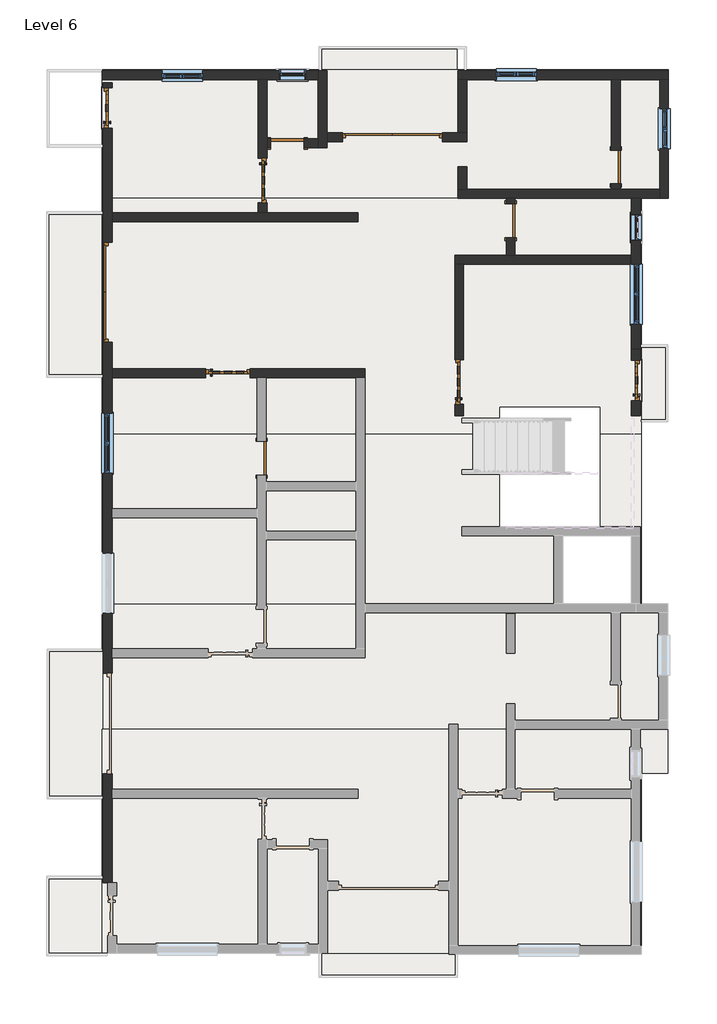
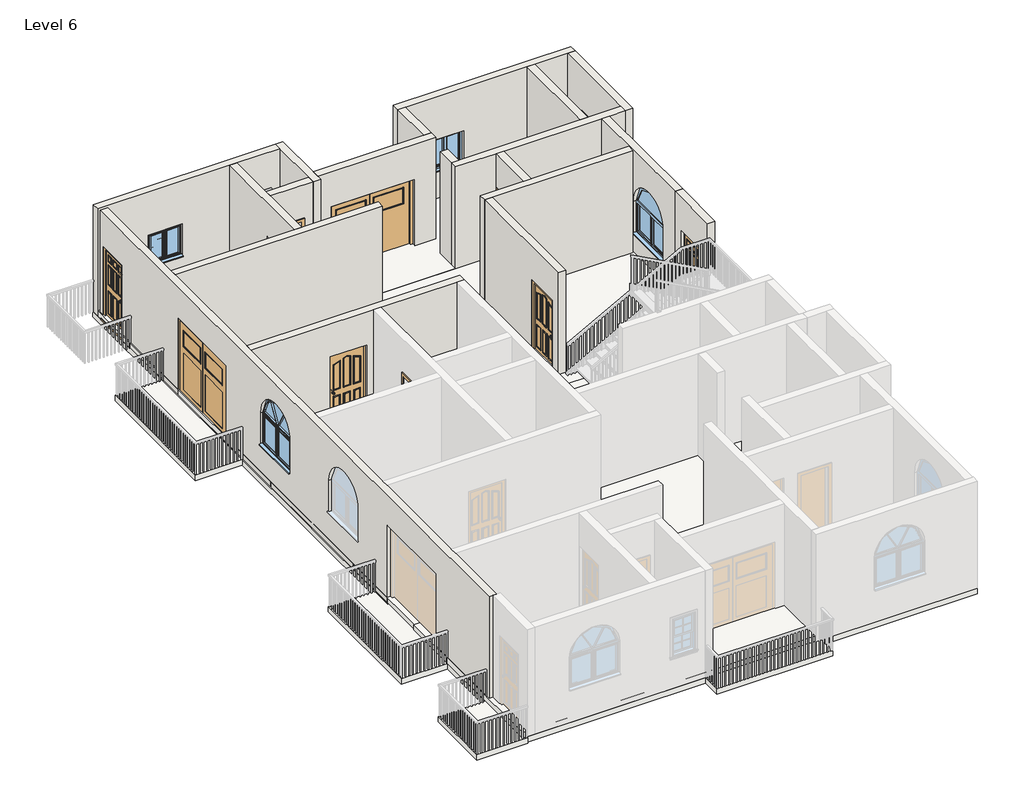
# One storey, part 2 of 7: 19 walls, 11 doors, 9 slabs, 7 windows, 5 roofs.
# Revit data of these elements (continued)
# Type "Windows_Dbl_w-Glazing_Bars : 910x910mm" (continued)
#   Frame Depth = 0' - 2.55906"
#   Default Head Height = 6' - 10.67717"
#   Cill Depth = 0' - 3.44488"
#   Cavity Closer Width = 0' - 1.9685"
#   Cavity Closer Offset from Ext = 0' - 4.03543"
#   Cavity Closer Depth = 0' - 3.34646"
#   Vis - Glazing Bars = yes
#   Vis - Cavity Closers = yes
#   Define Thermal Properties by = 1
#   Material Trim = Window Frame
#   Material Glazing Bars = Window Frame
#   Material Glass = Glass
#   Material Frame = Window Frame
#   Wall Closure = (empty or 0)
# Elements 1, 2 (IfcDoor, "Doors_ExtSgl_5 : 910x2110mm")
#   Phase Created = New Construction
#   Materials on its faces: "Door - Panel", "Door - Handle", "Door - Frame/Mullion", "Door - Glazing"
# Elements 3, 4, 5 (IfcDoor, "Doors_ExtSgl_6 : 1010x2110mm")
#   Phase Created = New Construction
#   Materials on its faces: "Door - Panel", "Door - Handle", "Door - Frame/Mullion", "Door - Glazing"
# Element 6 (IfcDoor, "Doors_Garage_Timber_Side_Hung_Glazing : 2270x2050mm")
#   Phase Created = New Construction
#   Materials on its faces: "Door - Panel", "Door - Frame/Mullion", "Door - Glazing"
# Element 7 (IfcDoor, "Doors_Garage_Timber_Side_Hung_Glazing : 2270x2200mm")
#   Phase Created = New Construction
#   Materials on its faces: "Door - Panel", "Door - Frame/Mullion", "Door - Glazing"
# Elements 8, 9, 10, 11 (IfcDoor, "Single-Flush : 30\" x 80\"")
#   Phase Created = New Construction
#   Materials on its faces: "Door - Frame", "Door - Panel"
# Elements 12, 16 (IfcRoof, "Generic - 12\"")
#   built-in parameter 1001705 = 50.5 (stored number, unit not read)
#   built-in parameter 1001710 = 33615
#   Phase Created = New Construction
#   Materials on its faces: "Default Roof", "Earth"
# Element 13 (IfcRoof, "Generic - 12\"")
#   built-in parameter 1001705 = 50.5 (stored number, unit not read)
#   built-in parameter 1001710 = 33615
#   Phase Created = New Construction
#   Materials on its faces: "Default Roof"
# Element 14 (IfcRoof, "Generic - 12\"")
#   built-in parameter 1001705 = 50.5 (stored number, unit not read)
#   built-in parameter 1001710 = 33615
#   Phase Created = New Construction
#   Materials on its faces: "Default Roof", "Concrete, Lightweight"
# Element 15 (IfcRoof, "Generic - 12\"")
#   built-in parameter 1001705 = 50.5 (stored number, unit not read)
#   built-in parameter 1001710 = 33615
#   Phase Created = New Construction
#   Materials on its faces: "Default Roof", "Wood - Stained"
# Element 17 (IfcSlab, "Generic - 12\"")
#   Height Offset From Level = 0' - 0"
#   Phase Created = New Construction
#   Materials on its faces: "Default Floor", "Concrete, Lightweight"
# Element 18 (IfcSlab, "Generic - 12\"")
#   Height Offset From Level = 0' - 0"
#   Phase Created = New Construction
#   Materials on its faces: "Default Floor", "Wood - Stained", "Earth"
# Elements 19, 21, 22, 23, 24 (IfcSlab, "Generic - 12\"")
#   Height Offset From Level = 0' - 0"
#   Phase Created = New Construction
#   Materials on its faces: "Default Floor"
# Element 20 (IfcSlab, "Generic - 12\"")
#   Height Offset From Level = 0' - 0"
#   Phase Created = New Construction
#   Materials on its faces: "Default Floor", "mm", "Brick, Soldier Course"
# Element 25 (IfcSlab, "Generic - 12\"")
#   Height Offset From Level = 0' - 0"
#   Phase Created = New Construction
#   Materials on its faces: "Default Floor", "Earth", "Concrete, Lightweight"
# Elements 26, 30 (IfcWall, "Generic - 9\" w")
#   Top Offset = 0' - 0"
#   Base Offset = 0' - 0"
#   wall height = 10' - 0"
#   Phase Created = New Construction
#   Base Constraint = Level 6
#   Top Constraint = Level 7
#   Materials on its faces: "Default Wall", "Earth"
# Element 27 (IfcWall, "Generic - 9\" w")
#   Top Offset = 0' - 0"
#   Base Offset = 0' - 0"
#   wall height = 10' - 0"
#   Phase Created = New Construction
#   Base Constraint = Level 6
#   Top Constraint = Level 7
#   Materials on its faces: "Default Wall", "Wood - Stained"
# Element 28 (IfcWall, "Generic - 9\" w")
#   Top Offset = 0' - 0"
#   Base Offset = 0' - 0"
#   wall height = 10' - 0"
#   Phase Created = New Construction
#   Base Constraint = Level 6
#   Top Constraint = Level 7
#   Materials on its faces: "Default Wall", "Grass"
# Element 29 (IfcWall, "Generic - 9\" w")
#   Top Offset = 0' - 0"
#   Base Offset = 0' - 0"
#   wall height = 10' - 0"
#   Phase Created = New Construction
#   Base Constraint = Level 6
#   Top Constraint = Level 7
#   Materials on its faces: "Default Wall", "mm"
# Elements 31, 32, 34, 36, 37, 39, 40, 41, 42, 43, 44 (IfcWall, "Generic -4.5\" p")
#   Top Offset = 0' - 0"
#   Base Offset = 0' - 0"
#   wall height = 10' - 0"
#   Phase Created = New Construction
#   Base Constraint = Level 6
#   Top Constraint = Level 7
#   Materials on its faces: "Default Wall"
# Elements 33, 38 (IfcWall, "Generic -4.5\" p")
#   Top Offset = 0' - 0"
#   Base Offset = 0' - 0"
#   wall height = 10' - 0"
#   Phase Created = New Construction
#   Base Constraint = Level 6
#   Top Constraint = Level 7
#   Materials on its faces: "Default Wall", "Earth"
# Element 35 (IfcWall, "Generic -4.5\" p")
#   Top Offset = 0' - 0"
#   Base Offset = 0' - 0"
#   wall height = 10' - 0"
#   Phase Created = New Construction
#   Base Constraint = Level 6
#   Top Constraint = Level 7
#   Materials on its faces: "Default Wall", "Oak Flooring"
# Element 45 (IfcWindow, "Window-Double-Hung : 24\" x 42\"")
#   Mark = "72"
#   Window Inset = 0' - 0"
#   Interior Wall Closure = 0' - 1 1/2"
#   Frame Extension = 0' - 1 1/4"
#   Exterior Wall Closure = 0' - 0 1/2"
#   Interior Trim Visibility = yes
#   Indicator Visibility = yes
#   Exterior Trim Visibility = yes
#   Phase Created = New Construction
#   Materials on its faces: "Wood - Stained", "Glass", "Clad - White"
# Element 46 (IfcWindow, "Window-Double-Hung : 24\" x 42\"")
#   Mark = "78"
#   Window Inset = 0' - 0"
#   Interior Wall Closure = 0' - 1 1/2"
#   Frame Extension = 0' - 1 1/4"
#   Exterior Wall Closure = 0' - 0 1/2"
#   Interior Trim Visibility = yes
#   Indicator Visibility = yes
#   Exterior Trim Visibility = yes
#   Phase Created = New Construction
#   Materials on its faces: "Wood - Stained", "Glass", "Clad - White"
# Element 47 (IfcWindow, "Windows_Arched : 1360x910mm")
#   Mark = "68"
#   Phase Created = New Construction
#   Materials on its faces: "Window Frame", "Glass"
# Element 48 (IfcWindow, "Windows_Arched : 1360x910mm")
#   Mark = "79"
#   Phase Created = New Construction
#   Materials on its faces: "Window Frame", "Glass"
# Element 49 (IfcWindow, "Windows_Dbl_w-Glazing_Bars : 910x910mm")
#   Mark = "75"
#   Phase Created = New Construction
#   Materials on its faces: "Window Frame", "Glass"
# Element 50 (IfcWindow, "Windows_Dbl_w-Glazing_Bars : 910x910mm")
#   Mark = "76"
#   Phase Created = New Construction
#   Materials on its faces: "Window Frame", "Glass"
# Element 51 (IfcWindow, "Windows_Dbl_w-Glazing_Bars : 910x910mm")
#   Mark = "77"
#   Phase Created = New Construction
#   Materials on its faces: "Window Frame", "Glass"
# Materials
#   "Door - Glazing": colour RGB 0 0 255, transparency 0.75
#   "Door - Panel": class "Wood", colour RGB 210 159 95, transparency 0, Cost = 0
#   "Door - Frame/Mullion": class "Wood", colour RGB 212 179 113, transparency 0
#   "Door - Handle": colour RGB 0 0 0, transparency 0
#   "Door - Frame": colour RGB 118 70 51, transparency 0, Cost = 0
#   "Wood - Stained": class "Wood", colour RGB 224 178 126, transparency 0, Cost = 0
#   "Clad - White": class "Wood", colour RGB 242 242 238, transparency 0, Cost = 0
#   "Glass": class "Glass", colour RGB 0 128 192, transparency 0.75, Description = "Soda Lime Glass", Cost = 0
#   "Window Frame": colour RGB 249 249 249, transparency 0
#   "Default Roof": colour RGB 88 101 114, transparency 0, Cost = 0
#   "Earth": class "Generic", colour RGB 97 75 62, transparency 0, Description = "Soil", Cost = 0
#   "Concrete, Lightweight": class "Concrete", colour RGB 142 141 140, transparency 0, Description = "Lightweight concrete", Cost = 0
#   "Default Floor": colour RGB 128 128 128, transparency 0, Cost = 0
#   "mm": class "Generic", colour RGB 128 64 0, transparency 0.5, Cost = 0
#   "Brick, Soldier Course": class "Masonry", colour RGB 170 98 104, transparency 0, Description = "Common brick soldier coursed", Cost = 0
#   "Default Wall": colour RGB 128 128 128, transparency 0, Cost = 0
#   "Grass": class "Generic", colour RGB 104 137 66, transparency 0, Description = "Physical material.", Cost = 0
#   "Oak Flooring": class "Wood", colour RGB 216 169 114, transparency 0, Description = "Quercus Rubra", Cost = 0
